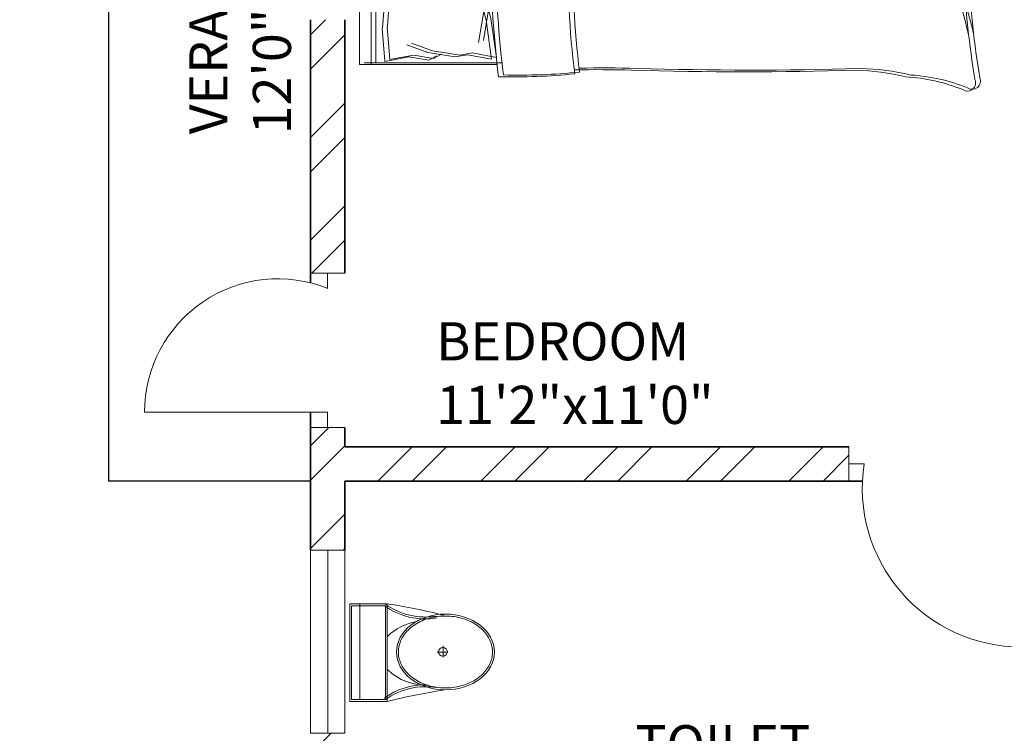
# Model space of a CAD drawing. Units: inches. Extents: x 1885 to 2748, y 783 to 2421.
# Tile 30 of 117: x 1969 to 2098, y 1350 to 1443. Entities that reach past the tile are written whole.
import ezdxf

# ---------------------------------------------------------------- set-up
doc = ezdxf.new("R2010")
doc.units = ezdxf.units.IN
for name, color, linetype, lineweight in [('A-ANNO-DIMS', 2, 'Continuous', 18), ('A-AREA-IDEN', 7, 'Continuous', 18), ('A-DOOR', 31, 'Continuous', 18), ('A-FLOR-BALC', 7, 'Continuous', 25), ('A-FLOR-FIXT', 8, 'Continuous', 18), ('A-FURN', 8, 'Continuous', 13), ('A-GLAZ', 181, 'Continuous', 18), ('A-WALL', 7, 'Continuous', 35)]:
    doc.layers.add(name, color=color, linetype=linetype, lineweight=lineweight)
doc.layers.add('A-WALL-PATT', color=85, linetype='Continuous', lineweight=13, true_color=0x58ba48)
doc.styles.get("Standard").update_dxf_attribs({"font": 'arial.ttf'})
doc.dimstyles.get("Standard").update_dxf_attribs({"dimtxt": 0.18, "dimasz": 0.18, "dimexe": 0.18, "dimexo": 0.0625, "dimgap": 0.09, "dimtad": 0, "dimtih": 1, "dimtoh": 1, "dimdec": 4, "dimzin": 0, "dimdsep": 46, "dimtxsty": 'Standard', "dimcen": 0.09, "dimadec": 0, "dimazin": 0, "dimtfac": 1, "dimtdec": 4, "dimtofl": 0, "dimtmove": 0, "dimatfit": 3, "dimfxl": 1, "dimtolj": 1, "dimtzin": 0, "dimarcsym": 0})

# ---------------------------------------------------------------- blocks, each defined once
blk = doc.blocks.new('A$C31115884')
for p, q in [((283.1, 497.7), (223.4, 497.7)), ((257.5, 466.4), (257.5, 523.2)), ((0, 200), (0, 0)), ((520, 200), (0, 200)), ((10, 190), (10, 10)), ((510, 190), (10, 190)), ((510, 10), (510, 190)), ((520, 0), (520, 200)), ((510, 54.5), (0, 54.5)), ((10, 10), (510, 10)), ((0, 0), (520, 0))]:
    blk.add_line(p, q)
blk.add_circle((255.6, 496.4), 23.6)
for centre, radius, start, end in [((2777.7, -204.6), 2807, 165.4549, 171.7133), ((3237, 905), 2807, 188.2867, 194.5451), ((-294.5, 403.3), 364.7, 324.2091, 9.3499), ((-294.5, 403.3), 374.7, 324.2091, 9.3499), ((139.5, 406.2), 293.5, 315.8436, 2.6563), ((805.8, 403.3), 364.7, 170.6501, 215.7909), ((805.8, 403.3), 374.7, 179.2036, 215.7909), ((383.6, 406.2), 293.5, 190.2774, 224.1564)]:
    blk.add_arc(centre, radius, start, end)
blk.add_ellipse((256.2, 509.9), major_axis=(0, -260.7), ratio=0.772727)
blk.add_open_spline([(256.2, 259.2), (263.1, 259.2), (270, 259.7), (287.8, 262.3), (298.7, 265.1), (319.9, 273.1), (330.2, 278.4), (350.1, 291.1), (359.7, 298.7), (377.7, 315.9), (386.2, 325.5), (401.7, 346.6), (408.8, 358.1), (421.3, 382.5), (426.8, 395.5), (435.9, 422.4), (439.5, 436.4), (444.8, 465.1), (446.5, 479.7), (447.9, 509.2), (447.6, 524), (445, 553.3), (442.7, 567.8), (436.3, 596), (432.1, 609.7), (421.9, 636), (416, 648.6), (402.5, 672.1), (395, 683), (378.6, 703), (369.8, 712.1), (351.1, 728), (341.3, 734.8), (320.9, 746.2), (310.4, 750.7), (288.9, 757.3), (278, 759.4), (256, 761), (245, 760.6), (223.1, 757.2), (212.3, 754.3), (191.1, 746.1), (180.8, 740.7), (160.9, 727.8), (151.4, 720.1), (133.5, 702.7), (125.1, 693), (109.6, 671.7), (102.6, 660.2), (90.2, 635.7), (84.9, 622.7), (76, 595.6), (72.4, 581.6), (67.2, 552.9), (65.6, 538.2), (64.4, 508.8), (64.8, 494), (67.5, 464.7), (69.9, 450.2), (76.6, 422), (80.8, 408.3), (91.1, 382.2), (97.2, 369.7), (110.8, 346.3), (118.4, 335.4), (134.8, 315.6), (143.7, 306.7), (162.4, 290.9), (172.3, 284.2), (192.8, 273), (203.3, 268.6), (224.8, 262.2), (235.8, 260.2), (249.9, 259.3), (253, 259.2), (256.2, 259.2)], degree=3, knots=[0, 0, 0, 0, 0.110105, 0.110105, 0.285049, 0.285049, 0.459994, 0.459994, 0.634938, 0.634938, 0.809882, 0.809882, 0.984827, 0.984827, 1.159771, 1.159771, 1.334715, 1.334715, 1.50966, 1.50966, 1.684604, 1.684604, 1.859549, 1.859549, 2.034493, 2.034493, 2.209437, 2.209437, 2.384382, 2.384382, 2.559326, 2.559326, 2.73427, 2.73427, 2.909215, 2.909215, 3.084159, 3.084159, 3.259103, 3.259103, 3.434048, 3.434048, 3.608992, 3.608992, 3.783936, 3.783936, 3.958881, 3.958881, 4.133825, 4.133825, 4.30877, 4.30877, 4.483714, 4.483714, 4.658658, 4.658658, 4.833603, 4.833603, 5.008547, 5.008547, 5.183491, 5.183491, 5.358436, 5.358436, 5.53338, 5.53338, 5.708324, 5.708324, 5.883269, 5.883269, 6.058213, 6.058213, 6.233158, 6.233158, 6.283185, 6.283185, 6.283185, 6.283185])
blk = doc.blocks.new('BED-DOUBLE')
for p, q in [((28.39, 53.09), (25.14, 49.39)), ((28.39, 53.09), (25.14, 49.39)), ((29.49, 52.95), (27.75, 52.87, 3.87)), ((29.49, 52.95), (27.75, 52.87, 3.87)), ((30.13, 53.17), (28.39, 53.09, 3.87)), ((30.13, 53.17), (28.39, 53.09, 3.87)), ((29.01, 51.56), (28.39, 53.09)), ((29.01, 51.56), (28.39, 53.09)), ((27.75, 52.87), (24.5, 49.16)), ((27.75, 52.87), (24.5, 49.16)), ((28.37, 51.33), (27.75, 52.87)), ((28.37, 51.33), (27.75, 52.87)), ((0, 51.49), (0.64, 51.49)), ((0, 3.47), (0, 51.49)), ((0, 51.26), (26.61, 51.26)), ((0, 51.26), (26.61, 51.26)), ((0.64, 51.49), (27.25, 51.49)), ((0.64, 51.49), (27.25, 51.49)), ((1.54, 3.47), (1.54, 51.26)), ((1.54, 3.47), (1.54, 51.26)), ((2.18, 3.7), (2.18, 51.49)), ((2.18, 3.7), (2.18, 51.49)), ((6.41, 49.96), (8.98, 50.56)), ((6.41, 49.96), (8.98, 50.56)), ((8.98, 50.56), (10.03, 50.04)), ((8.98, 50.56), (10.03, 50.04)), ((16.58, 50.7), (13.44, 49.92)), ((16.58, 50.7), (13.44, 49.92)), ((17.22, 50.93), (14.08, 50.15)), ((17.22, 50.93), (14.08, 50.15)), ((16.17, 45.57), (16.58, 50.7)), ((16.17, 45.56), (16.58, 50.7)), ((16.81, 45.79), (17.22, 50.93)), ((16.81, 45.79), (17.22, 50.93)), ((28.06, 48.23), (28.37, 51.33)), ((28.06, 48.23), (28.37, 51.33)), ((28.7, 48.46), (29.01, 51.56)), ((28.7, 48.46), (29.01, 51.56)), ((2.56, 50.11), (2.46, 44.71)), ((2.56, 50.11), (2.46, 44.71)), ((2.56, 50.11), (5.77, 49.73)), ((2.56, 50.11), (5.77, 49.73)), ((3.2, 50.34), (3.1, 44.94)), ((3.2, 50.34), (3.1, 44.94)), ((3.2, 50.34), (6.41, 49.96)), ((3.2, 50.34), (6.41, 49.96)), ((8.26, 49.31), (5.58, 48.13)), ((8.26, 49.31), (5.58, 48.13)), ((5.77, 49.73), (8.34, 50.33)), ((5.77, 49.73), (8.34, 50.33)), ((8.9, 49.54), (6.22, 48.36)), ((8.9, 49.54), (6.22, 48.36)), ((11.83, 50.11), (8.26, 49.31)), ((11.83, 50.11), (8.26, 49.31)), ((8.34, 50.33), (9.39, 49.81)), ((8.34, 50.33), (9.39, 49.81)), ((12.47, 50.34), (8.9, 49.54)), ((12.47, 50.34), (8.9, 49.54)), ((13.44, 49.92), (11.83, 50.11)), ((13.44, 49.92), (11.83, 50.11)), ((14.08, 50.15), (12.47, 50.34)), ((14.08, 50.15), (12.47, 50.34)), ((24.5, 49.16), (22.33, 46.22)), ((24.5, 49.16), (22.33, 46.22)), ((25.14, 49.39), (22.97, 46.45)), ((25.14, 49.39), (22.97, 46.45)), ((28.37, 44.36), (28.06, 48.23)), ((28.37, 44.36), (28.06, 48.23)), ((29.01, 44.59), (28.7, 48.46)), ((29.01, 44.59), (28.7, 48.46)), ((2.46, 44.71), (2.55, 45.71)), ((2.46, 44.71), (2.55, 45.71)), ((2.55, 45.71), (3.07, 41.91)), ((2.55, 45.71), (3.07, 41.91)), ((3.1, 44.94), (3.19, 45.94)), ((3.1, 44.94), (3.19, 45.94)), ((3.19, 45.94), (3.71, 42.14)), ((3.19, 45.94), (3.71, 42.14)), ((16.73, 43.6), (16.17, 45.57)), ((16.73, 43.6), (16.17, 45.56)), ((17.37, 43.83), (16.81, 45.79)), ((17.37, 43.83), (16.81, 45.79)), ((22.33, 46.22), (20.32, 40.64)), ((22.33, 46.22), (20.32, 40.64)), ((22.97, 46.45), (20.96, 40.87)), ((22.97, 46.45), (20.96, 40.87)), ((28.83, 40.95), (28.37, 44.36)), ((28.83, 40.95), (28.37, 44.36)), ((29.47, 41.18), (29.01, 44.59)), ((29.47, 41.18), (29.01, 44.59)), ((16.3, 36.59), (16.73, 43.6)), ((16.3, 36.59), (16.73, 43.6)), ((16.94, 36.82), (17.37, 43.83)), ((16.94, 36.82), (17.37, 43.83)), ((3.07, 41.91), (4.43, 36.49)), ((3.07, 41.91), (4.43, 36.49)), ((3.71, 42.14), (5.07, 36.72)), ((3.71, 42.14), (5.07, 36.72)), ((20.32, 40.64), (17.39, 32.3)), ((20.32, 40.64), (17.39, 32.3)), ((20.96, 40.87), (18.03, 32.53)), ((20.96, 40.87), (18.03, 32.53)), ((29.76, 38.94), (28.83, 40.95)), ((29.76, 38.94), (28.83, 40.95)), ((30.4, 39.17), (29.47, 41.18)), ((30.4, 39.17), (29.47, 41.18)), ((3.68, 39.2), (3.08, 37.13)), ((3.68, 39.2), (3.08, 37.13)), ((4.32, 39.43), (3.72, 37.36)), ((4.32, 39.43), (3.72, 37.36)), ((30.38, 36.46), (29.76, 38.94)), ((30.38, 36.46), (29.76, 38.94)), ((31.02, 36.69), (30.4, 39.17)), ((31.02, 36.69), (30.4, 39.17)), ((79.25, 15.06), (79.25, 39.68)), ((79.25, 15.06), (79.25, 39.68)), ((79.89, 15.29), (79.89, 39.9)), ((79.89, 15.29), (79.89, 39.9)), ((3.08, 37.13), (2.54, 34.2)), ((3.08, 37.13), (2.54, 34.2)), ((3.72, 37.36), (3.18, 34.43)), ((3.72, 37.36), (3.18, 34.43)), ((15.63, 32.56), (16.3, 36.59)), ((15.63, 32.56), (16.3, 36.59)), ((16.27, 32.79), (16.94, 36.82)), ((16.27, 32.79), (16.94, 36.82)), ((23.88, 34.45), (28.37, 36.15)), ((23.88, 34.45), (28.37, 36.15)), ((24.52, 34.68), (29.01, 36.38)), ((24.52, 34.68), (29.01, 36.38)), ((28.37, 36.15), (30.38, 36.46)), ((28.37, 36.15), (30.38, 36.46)), ((29.01, 36.38), (31.02, 36.69)), ((29.01, 36.38), (31.02, 36.69)), ((2.54, 34.2), (2.56, 33.88)), ((2.54, 34.2), (2.56, 33.88)), ((2.56, 33.88), (2.98, 29.45)), ((2.56, 33.88), (2.98, 29.45)), ((3.18, 34.43), (3.2, 34.11)), ((3.18, 34.43), (3.2, 34.11)), ((3.2, 34.11), (3.62, 29.68)), ((3.2, 34.11), (3.62, 29.68)), ((16.74, 30.75), (15.46, 33.82)), ((16.74, 30.75), (15.46, 33.82)), ((17.38, 30.98), (16.1, 34.05)), ((17.38, 30.98), (16.1, 34.05)), ((17.39, 30.26), (23.88, 34.45)), ((17.39, 30.26), (23.88, 34.45)), ((18.03, 30.49), (24.52, 34.68)), ((18.03, 30.49), (24.52, 34.68)), ((16.9, 28.3), (16.74, 30.75)), ((16.9, 28.3), (16.74, 30.75)), ((17.54, 28.52), (17.38, 30.98)), ((17.54, 28.52), (17.38, 30.98)), ((2.98, 29.45), (2.5, 27.98)), ((2.98, 29.45), (2.5, 27.98)), ((3.62, 29.68), (3.13, 28.2)), ((3.62, 29.68), (3.13, 28.2)), ((14.86, 28.36), (17.54, 28.52)), ((14.86, 28.36), (17.54, 28.52)), ((2.5, 27.98), (7.87, 27.73)), ((2.5, 27.98), (7.87, 27.73)), ((3.13, 28.2), (8.51, 27.96)), ((3.13, 28.2), (8.51, 27.96)), ((7.22, 26.56), (10.4, 27.14)), ((7.22, 26.56), (10.4, 27.14)), ((7.86, 26.79), (11.04, 27.37)), ((7.86, 26.79), (11.04, 27.37)), ((7.87, 27.73), (11.08, 27.35)), ((7.87, 27.73), (11.08, 27.35)), ((8.51, 27.96), (11.72, 27.58)), ((8.51, 27.96), (11.72, 27.58)), ((10.4, 27.14), (11.71, 27.14)), ((10.4, 27.14), (11.71, 27.14)), ((11.04, 27.37), (12.35, 27.37)), ((11.04, 27.37), (12.35, 27.37)), ((11.08, 27.35), (12.38, 27.43)), ((11.08, 27.35), (12.38, 27.43)), ((11.71, 27.14), (13.59, 26.56)), ((11.71, 27.14), (13.59, 26.56)), ((11.72, 27.58), (13.02, 27.66)), ((11.72, 27.58), (13.02, 27.66)), ((12.35, 27.37), (14.22, 26.79)), ((12.35, 27.37), (14.22, 26.79)), ((12.38, 27.43), (14.22, 28.13)), ((12.38, 27.43), (14.22, 28.13)), ((13.02, 27.66), (14.86, 28.36)), ((13.02, 27.66), (14.86, 28.36)), ((14.22, 28.13), (16.9, 28.3)), ((14.22, 28.13), (16.9, 28.3)), ((1.87, 25.98), (7.22, 26.56)), ((1.87, 25.98), (7.22, 26.56)), ((2.45, 24.54), (1.87, 25.98)), ((2.45, 24.54), (1.87, 25.98)), ((2.51, 26.21), (7.86, 26.79)), ((2.51, 26.21), (7.86, 26.79)), ((3.09, 24.76), (2.51, 26.21)), ((3.09, 24.76), (2.51, 26.21)), ((13.59, 26.56), (16.27, 26.56)), ((13.59, 26.56), (16.27, 26.56)), ((14.22, 26.79), (16.91, 26.79)), ((14.22, 26.79), (16.91, 26.79)), ((16.27, 26.56), (16.27, 24.1)), ((16.27, 26.56), (16.27, 24.1)), ((16.91, 26.79), (16.91, 24.33)), ((16.91, 26.79), (16.91, 24.33)), ((2.31, 20.09), (2.45, 24.54)), ((2.31, 20.09), (2.45, 24.54)), ((2.95, 20.32), (3.09, 24.76)), ((2.95, 20.32), (3.09, 24.76)), ((16.81, 19.61), (17.22, 24.74)), ((16.81, 19.61), (17.22, 24.74)), ((16.27, 24.1), (15.18, 20.96)), ((16.27, 24.1), (15.18, 20.96)), ((16.91, 24.33), (15.82, 21.19)), ((16.91, 24.33), (15.82, 21.19)), ((16.17, 19.38), (16.58, 24.51)), ((16.17, 19.38), (16.58, 24.51)), ((2.31, 19.77), (2.31, 20.09)), ((2.31, 19.77), (2.31, 20.09)), ((3.03, 16.88), (2.31, 19.77)), ((3.03, 16.88), (2.31, 19.77)), ((2.95, 20), (2.95, 20.32)), ((2.95, 20), (2.95, 20.32)), ((3.67, 17.11), (2.95, 20)), ((3.67, 17.11), (2.95, 20)), ((16.73, 17.42), (16.17, 19.38)), ((16.73, 17.42), (16.17, 19.38)), ((17.37, 17.65), (16.81, 19.61)), ((17.37, 17.65), (16.81, 19.61)), ((3.75, 14.85), (3.03, 16.88)), ((3.75, 14.85), (3.03, 16.88)), ((3.32, 12.11), (4.33, 17.6)), ((3.32, 12.11), (4.33, 17.6)), ((4.39, 15.08), (3.67, 17.11)), ((4.39, 15.08), (3.67, 17.11)), ((3.96, 12.34), (4.97, 17.83)), ((3.96, 12.34), (4.97, 17.83)), ((16.3, 10.41), (16.73, 17.42)), ((16.3, 10.41), (16.73, 17.42)), ((16.94, 10.64), (17.37, 17.65)), ((16.94, 10.64), (17.37, 17.65)), ((3.03, 8.28), (3.32, 12.11)), ((3.03, 8.28), (3.32, 12.11)), ((3.67, 8.51), (3.96, 12.34)), ((3.67, 8.51), (3.96, 12.34)), ((15.63, 6.38), (16.3, 10.41)), ((15.63, 6.38), (16.3, 10.41)), ((16.27, 6.61), (16.94, 10.64)), ((16.27, 6.61), (16.94, 10.64)), ((16.3, 10.41), (16.62, 9.28)), ((16.3, 10.41), (16.62, 9.28)), ((16.94, 10.64), (17.26, 9.51)), ((16.94, 10.64), (17.26, 9.51)), ((16.62, 9.28), (17.34, 4.18)), ((16.62, 9.28), (17.34, 4.18)), ((17.26, 9.51), (17.98, 4.41)), ((17.26, 9.51), (17.98, 4.41)), ((3.01, 8.18), (3.03, 8.28)), ((3.01, 8.18), (3.03, 8.28)), ((3.34, 3.9), (3.01, 8.18)), ((3.34, 3.9), (3.01, 8.18)), ((3.65, 8.41), (3.67, 8.51)), ((3.65, 8.41), (3.67, 8.51)), ((3.98, 4.13), (3.65, 8.41)), ((3.98, 4.13), (3.65, 8.41)), ((8.96, 5.05), (6.21, 6.06)), ((8.96, 5.05), (6.21, 6.06)), ((9.6, 5.28), (6.85, 6.29)), ((9.6, 5.28), (6.85, 6.29)), ((13.21, 4.7), (9.6, 5.28)), ((13.21, 4.7), (9.6, 5.28)), ((3.32, 3.89), (6.5, 4.47)), ((3.32, 3.89), (6.5, 4.47)), ((3.96, 4.12), (7.14, 4.7)), ((3.96, 4.12), (7.14, 4.7)), ((6.5, 4.47), (9.1, 4.04)), ((6.5, 4.47), (9.1, 4.04)), ((7.14, 4.7), (9.74, 4.27)), ((7.14, 4.7), (9.74, 4.27)), ((12.57, 4.47), (8.96, 5.05)), ((12.57, 4.47), (8.96, 5.05)), ((9.1, 4.04), (10.12, 4.62)), ((9.1, 4.04), (10.12, 4.62)), ((9.74, 4.27), (10.75, 4.84)), ((9.74, 4.27), (10.75, 4.84)), ((14.16, 4.76), (12.57, 4.47)), ((14.16, 4.76), (12.57, 4.47)), ((14.8, 4.99), (13.21, 4.7)), ((14.8, 4.99), (13.21, 4.7)), ((17.34, 4.18), (14.16, 4.76)), ((17.34, 4.18), (14.16, 4.76)), ((17.98, 4.41), (14.8, 4.99)), ((17.98, 4.41), (14.8, 4.99)), ((18.11, 3.47), (0, 3.47)), ((18.11, 3.47), (0, 3.47)), ((18.75, 3.7), (0.64, 3.7)), ((18.75, 3.7), (0.64, 3.7))]:
    blk.add_line(p, q)
for centre, radius, start, end in [((69.31, 76.38), 23.07, 267.4714, 296.4681), ((69.31, 76.38), 23.07, 267.4714, 296.4681), ((79.51, 54.64), 1.1, 332.6588, 86.02), ((79.51, 54.64), 1.1, 332.6588, 86.02), ((68.67, 76.16), 23.07, 267.4714, 296.4681), ((68.67, 76.16), 23.07, 267.4714, 296.4681), ((78.87, 54.41), 1.1, 332.6588, 86.02), ((78.87, 54.41), 1.1, 332.6588, 86.02), ((-6.65, 51.33), 36.18, 349.8763, 2.5657), ((-6.65, 51.33), 36.18, 349.8763, 2.5657), ((36.32, 182.26), 129.5, 266.9791, 273.8365), ((36.32, 182.26), 129.5, 266.9791, 273.8365), ((-6.01, 51.55), 36.18, 349.8763, 2.5657), ((-6.01, 51.55), 36.18, 349.8763, 2.5657), ((36.96, 182.49), 129.5, 266.9791, 273.8365), ((36.96, 182.49), 129.5, 266.9791, 273.8365), ((67.83, -4508.74), 4561.86, 90.00217, 90.28689), ((67.83, -4508.75), 4561.86, 90.00217, 90.28689), ((68.46, -4508.52), 4561.86, 90.00217, 90.28689), ((68.46, -4508.52), 4561.86, 90.00217, 90.28689), ((212.28, 41.15), 133.04, 174.4998, 180.6351), ((212.28, 41.15), 133.04, 174.4998, 180.6351), ((212.92, 41.38), 133.04, 174.4998, 180.6351), ((212.92, 41.38), 133.04, 174.4998, 180.6351), ((35.71, 43.97), 6.22, 168.6608, 203.7384), ((35.71, 43.97), 6.22, 168.6608, 203.7384), ((35.07, 43.74), 6.22, 168.6608, 203.7384), ((35.07, 43.74), 6.22, 168.6608, 203.7384), ((2.13, 31.38), 29.65, 10.6617, 19.8806), ((2.13, 31.38), 29.65, 10.6617, 19.8806), ((1.49, 31.15), 29.65, 10.6617, 19.8806), ((1.49, 31.15), 29.65, 10.6617, 19.8806), ((156.32, 17.75), 129.02, 171.7845, 186.9006), ((156.32, 17.75), 129.02, 171.7845, 186.9006), ((156.96, 17.98), 129.02, 171.7845, 186.9006), ((156.96, 17.98), 129.02, 171.7845, 186.9006), ((30.44, 36.64), 0.185, 250.2464, 1.1377), ((30.44, 36.63), 0.185, 250.2464, 1.1377), ((31.08, 36.86), 0.185, 250.2464, 1.1377), ((31.08, 36.86), 0.185, 250.2464, 1.1377), ((182.06, 21.36), 164.97, 176.0865, 186.7821), ((182.06, 21.36), 164.97, 176.0865, 186.7821), ((182.7, 21.59), 164.97, 176.0865, 186.7821), ((182.7, 21.59), 164.97, 176.0865, 186.7821), ((-23.71, -17.22), 106.46, 13.3832, 17.7053), ((-23.71, -17.22), 106.46, 13.3832, 17.7053), ((-23.07, -16.99), 106.46, 13.3832, 17.7053), ((-23.07, -16.99), 106.46, 13.3832, 17.7053), ((200.84, 21.43), 121.76, 182.9958, 189.4091), ((200.84, 21.43), 121.76, 182.9958, 189.4091), ((201.48, 21.65), 121.76, 182.9958, 189.4091), ((201.48, 21.65), 121.76, 182.9958, 189.4091), ((31.18, -167.31), 170.11, 88.4762, 91.0082), ((31.18, -167.31), 170.11, 88.4762, 91.0082), ((31.82, -167.08), 170.11, 88.4762, 91.0082), ((31.82, -167.08), 170.11, 88.4762, 91.0082), ((50.62, 484.82), 482.31, 268.2277, 271.7185), ((50.62, 484.82), 482.31, 268.2277, 271.7185), ((51.26, 485.05), 482.31, 268.2277, 271.7185), ((51.26, 485.05), 482.31, 268.2277, 271.7185), ((64.52, -26.9), 29.63, 76.0648, 88.9113), ((64.52, -26.9), 29.63, 76.0648, 88.9113), ((65.16, -26.67), 29.63, 76.0648, 88.9113), ((65.16, -26.67), 29.63, 76.0648, 88.9113), ((20.1, 85.16), 83.31, 268.7218, 275.604), ((20.1, 85.16), 83.31, 268.7218, 275.604), ((20.74, 85.39), 83.31, 268.7218, 275.604), ((20.74, 85.39), 83.31, 268.7218, 275.604), ((70.28, -21.66), 23.56, 67.9751, 86.652), ((70.28, -21.66), 23.56, 67.9751, 86.652), ((70.92, -21.43), 23.56, 67.9751, 86.652), ((70.92, -21.43), 23.56, 67.9751, 86.652), ((79.72, 1.09), 1.09, 236.1736, 23.4781), ((79.72, 1.09), 1.09, 236.1736, 23.4781), ((80.36, 1.31), 1.09, 236.1736, 23.4781), ((80.36, 1.31), 1.09, 236.1736, 23.4781)]:
    blk.add_arc(centre, radius, start, end)
blk = doc.blocks.new('WIN-24')
for p, q in [((0, 4.5), (0, 0)), ((0, 4.5), (24, 4.5)), ((24, 2.25), (24, 4.5)), ((24, 4.5), (24, 0)), ((0, 0), (0, 2.25)), ((0, 2.25), (24, 2.25)), ((24, 0), (0, 0))]:
    blk.add_line(p, q)
blk = doc.blocks.new('*D45')
at = {"layer": 'A-ANNO-DIMS', "color": 0, "lineweight": -2, "transparency": 16777216}
for p, q in [((1980.71, 1524.01), (1902.84, 1524.01)), ((1903.02, 1523.83), (1903.02, 1290.94)), ((1903.02, 1057.69), (1903.02, 1290.57)), ((1971.21, 1057.51), (1902.84, 1057.51))]:
    blk.add_line(p, q, dxfattribs=at)
at = {"layer": 'A-ANNO-DIMS', "color": 0, "transparency": 16777216}
for points in [[(1902.99, 1523.83), (1903.05, 1523.83), (1903.02, 1524.01)], [(1902.99, 1057.69), (1903.05, 1057.69), (1903.02, 1057.51)]]:
    blk.add_solid(points, dxfattribs=at)
at = {"layer": 'Defpoints', "color": 0, "transparency": 16777216}
for p in [(1903.02, 1524.01), (1980.77, 1524.01), (1971.27, 1057.51)]:
    blk.add_point(p, dxfattribs=at)
at = {"layer": 'A-ANNO-DIMS', "color": 0, "transparency": 16777216, "insert": (1903.02, 1290.76), "char_height": 0.18, "attachment_point": 5}
blk.add_mtext('\\A1;466.5', dxfattribs=at)

msp = doc.modelspace()

# ---------------------------------------------------------------- hatches: boundary and pattern name
at = {"layer": 'A-WALL-PATT'}
h = msp.add_hatch(dxfattribs=at)
h.set_pattern_fill('ANSI32', color=256)
h.paths.add_polyline_path([(2007.77, 2318.01), (1980.77, 2318.01), (1980.77, 2281.22), (1985.27, 2281.22), (1985.27, 2313.51), (2007.77, 2313.51), (2007.77, 2315.76)])
h.paths.add_polyline_path([(2094.32, 2318.01), (2067.77, 2318.01), (2067.77, 2313.51), (2094.32, 2313.51), (2094.32, 2315.76)])
h.paths.add_polyline_path([(2131.37, 2315.76), (2131.37, 2318.01), (2131.19, 2318.01), (2112.61, 2318.01), (2112.61, 2313.51), (2117.27, 2313.51), (2117.27, 2255.2), (2121.77, 2255.2), (2121.77, 2313.51), (2131.37, 2313.51)])
h.paths.add_polyline_path([(2190.51, 2318.01), (2155.37, 2318.01), (2155.37, 2313.51), (2169.77, 2313.51), (2169.77, 2229.51), (2121.77, 2229.51), (2121.77, 2233.45), (2119.52, 2233.45), (2117.27, 2233.45), (2117.27, 2201.1), (2121.77, 2201.1), (2121.77, 2225.01), (2169.77, 2225.01), (2169.77, 2165.01), (2306.27, 2165.01), (2306.27, 2066.01), (2310.77, 2066.01), (2344.27, 2066.01), (2486.27, 2066.01), (2486.27, 1886.01), (2483.02, 1886.01), (2483.02, 1881.51), (2486.27, 1881.51), (2486.27, 1880.68), (2490.77, 1880.68), (2490.77, 2070.51), (2344.27, 2070.51), (2310.77, 2070.51), (2310.77, 2165.01), (2310.77, 2173.64), (2308.52, 2173.64), (2306.27, 2173.64), (2306.27, 2169.51), (2174.27, 2169.51), (2174.27, 2313.51), (2190.51, 2313.51), (2190.51, 2315.76)])
h.paths.add_polyline_path([(1985.27, 2221.22), (1980.77, 2221.22), (1980.77, 2165.01), (1992.77, 2165.01), (1992.77, 2141.93), (1997.27, 2141.93), (1997.27, 2165.01), (2117.27, 2165.01), (2117.27, 2163.13), (2121.77, 2163.13), (2121.77, 2172.73), (2119.52, 2172.73), (2117.27, 2172.73), (2117.27, 2169.51), (1985.27, 2169.51)])
h.paths.add_polyline_path([(1997.27, 2105.93), (1992.77, 2105.93), (1992.77, 2070.51), (2016.77, 2070.51), (2016.77, 2059.12), (2019.02, 2059.12), (2021.27, 2059.12), (2021.27, 2070.51), (2117.27, 2070.51), (2117.27, 2022.51), (2114.42, 2022.51), (2114.42, 2018.01), (2123.63, 2018.01), (2123.63, 2020.26), (2123.63, 2022.51), (2121.77, 2022.51), (2121.77, 2142.59), (2119.52, 2142.59), (2117.27, 2142.59), (2117.27, 2075.01), (1997.27, 2075.01)])
h.paths.add_polyline_path([(2092.03, 2020.26), (2092.03, 2022.51), (2021.27, 2022.51), (2021.27, 2035.12), (2016.77, 2035.12), (2016.77, 2018.01), (2016.77, 1978.78), (2021.27, 1978.78), (2021.27, 2018.01), (2092.03, 2018.01)])
h.paths.add_polyline_path([(2260.94, 2022.51), (2153.1, 2022.51), (2153.1, 2020.26), (2153.1, 2018.01), (2155.27, 2018.01), (2155.27, 1886.01), (2107.63, 1886.01), (2107.63, 1881.51), (2182.91, 1881.51), (2182.91, 1883.76), (2182.91, 1886.01), (2159.77, 1886.01), (2159.77, 2018.01), (2260.94, 2018.01), (2260.94, 2020.26)])
h.paths.add_polyline_path([(2047.63, 1883.76), (2047.63, 1886.01), (2021.27, 1886.01), (2021.27, 1918.78), (2019.02, 1918.78), (2016.77, 1918.78), (2016.77, 1881.51), (2047.63, 1881.51)])
h.paths.add_polyline_path([(2306.36, 1883.76), (2306.36, 1886.01), (2296.27, 1886.01), (2296.27, 1982.01), (2316.54, 1982.01), (2316.54, 1984.26), (2316.54, 1986.51), (2296.27, 1986.51), (2296.27, 2022.51), (2289.28, 2022.51), (2289.28, 2018.01), (2291.77, 2018.01), (2291.77, 1886.01), (2242.91, 1886.01), (2242.91, 1881.51), (2306.36, 1881.51)], flags=17)
h.paths.add_polyline_path([(1985.27, 1843.01), (2021.6, 1843.01), (2021.53, 1845.44), (2021.48, 1847.51), (1980.77, 1847.51), (1980.77, 1809.45), (1985.27, 1809.45)])
h.paths.add_polyline_path([(2131.48, 1845.26), (2131.48, 1847.51), (2081.53, 1847.51), (2081.53, 1843.01), (2117.27, 1843.01), (2117.27, 1784.15), (2119.52, 1784.15), (2121.77, 1784.15), (2121.77, 1843.01), (2131.48, 1843.01)])
h.paths.add_polyline_path([(2203.89, 1847.51), (2155.48, 1847.51), (2155.48, 1843.01), (2169.77, 1843.01), (2169.77, 1759.01), (2121.77, 1759.01), (2121.77, 1761.46), (2117.27, 1761.46), (2117.27, 1730.43), (2121.77, 1730.43), (2121.77, 1754.51), (2177.42, 1754.51), (2177.42, 1756.76), (2177.42, 1759.01), (2174.27, 1759.01), (2174.27, 1843.01), (2203.89, 1843.01)])
h.paths.add_polyline_path([(2335.55, 1845.26), (2335.55, 1847.51), (2239.89, 1847.51), (2239.89, 1843.01), (2306.27, 1843.01), (2306.27, 1759.01), (2199.49, 1759.01), (2199.49, 1754.51), (2310.77, 1754.51), (2310.77, 1843.01), (2335.55, 1843.01)])
h.paths.add_polyline_path([(2348.77, 2022.51), (2344.27, 2022.51), (2344.27, 1986.51), (2341.68, 1986.51), (2341.68, 1982.01), (2344.27, 1982.01), (2344.27, 1886.01), (2330.36, 1886.01), (2330.36, 1881.51), (2361.63, 1881.51), (2361.63, 1883.76), (2361.63, 1886.01), (2348.77, 1886.01)], flags=17)
h.paths.add_polyline_path([(2283.25, 2315.76), (2283.25, 2318.01), (2238.51, 2318.01), (2238.51, 2313.51), (2283.25, 2313.51)], flags=17)
h.paths.add_polyline_path([(2363.27, 2348.01), (2388.68, 2348.01), (2388.68, 2350.26), (2388.68, 2352.51), (2358.77, 2352.51), (2358.77, 2348.01), (2358.77, 2318.01), (2344.48, 2318.01), (2344.48, 2313.51), (2358.77, 2313.51), (2358.77, 2229.51), (2310.77, 2229.51), (2310.77, 2231.95), (2306.27, 2231.95), (2306.27, 2205.61), (2310.77, 2205.61), (2310.77, 2225.01), (2358.77, 2225.01), (2358.77, 2211.51), (2452.33, 2211.51), (2452.33, 2213.76), (2452.33, 2216.01), (2363.27, 2216.01), (2363.27, 2318.01)])
h.paths.add_polyline_path([(2310.77, 2313.51), (2320.48, 2313.51), (2320.48, 2315.76), (2320.48, 2318.01), (2302.73, 2318.01), (2302.73, 2313.51), (2306.27, 2313.51), (2306.27, 2251.08), (2310.77, 2251.08)], flags=17)
h.paths.add_polyline_path([(2490.77, 2352.51), (2486.27, 2352.51), (2448.68, 2352.51), (2448.68, 2348.01), (2486.27, 2348.01), (2486.27, 2318.01), (2486.27, 2216.01), (2481.78, 2216.01), (2481.78, 2211.51), (2486.27, 2211.51), (2486.27, 2165.01), (2493.29, 2165.01), (2493.29, 2167.26), (2493.29, 2169.51), (2490.77, 2169.51), (2490.77, 2313.51), (2494.43, 2313.51), (2494.43, 2318.01), (2490.77, 2318.01)])
h.paths.add_polyline_path([(2534.65, 2318.01), (2515.69, 2318.01), (2515.69, 2313.51), (2534.65, 2313.51), (2534.65, 2315.76)])
h.paths.add_polyline_path([(2618.27, 2318.01), (2594.65, 2318.01), (2594.65, 2313.51), (2613.77, 2313.51), (2613.77, 2281.71), (2618.27, 2281.71)])
h.paths.add_polyline_path([(2618.27, 2221.71), (2613.77, 2221.71), (2613.77, 2169.51), (2554.02, 2169.51), (2554.02, 2165.01), (2613.77, 2165.01), (2613.77, 2152.88), (2618.27, 2152.88)])
h.paths.add_polyline_path([(2618.27, 2128.88), (2616.02, 2128.88), (2613.77, 2128.88), (2613.77, 2117.01), (2529.77, 2117.01), (2529.77, 2165.01), (2532.85, 2165.01), (2532.85, 2169.51), (2522.87, 2169.51), (2522.87, 2165.01), (2525.27, 2165.01), (2525.27, 2117.01), (2525.27, 2112.51), (2525.27, 2108.58), (2529.77, 2108.58), (2529.77, 2112.51), (2613.77, 2112.51), (2613.77, 2080.19), (2618.27, 2080.19)])
h.paths.add_polyline_path([(2618.27, 2044.19), (2616.02, 2044.19), (2613.77, 2044.19), (2613.77, 2015.51), (2529.77, 2015.51), (2529.77, 2088.58), (2527.52, 2088.58), (2525.27, 2088.58), (2525.27, 2011.01), (2613.77, 2011.01), (2613.77, 1956.75), (2618.27, 1956.75)])
h.paths.add_polyline_path([(2618.27, 1881.51), (2618.27, 1896.75), (2613.77, 1896.75), (2613.77, 1881.51), (2613.77, 1847.51), (2592.71, 1847.51), (2592.71, 1843.01), (2613.77, 1843.01), (2613.77, 1765.01), (2613.77, 1760.51), (2609.62, 1760.51), (2609.62, 1756.01), (2613.77, 1756.01), (2613.77, 1660.01), (2608.54, 1660.01), (2608.54, 1655.51), (2613.77, 1655.51), (2613.77, 1508.16), (2618.27, 1508.16)])
h.paths.add_polyline_path([(2565.77, 1843.01), (2569, 1843.01), (2569, 1847.51), (2490.77, 1847.51), (2490.77, 1849.7), (2488.52, 1849.7), (2486.27, 1849.7), (2486.27, 1847.51), (2477.27, 1847.51), (2477.27, 1838.51), (2477.27, 1821.49), (2486.27, 1821.49), (2486.27, 1838.51), (2561.27, 1838.51), (2561.27, 1765.01), (2486.27, 1765.01), (2486.27, 1786.16), (2477.27, 1786.16), (2477.27, 1765.01), (2477.27, 1756.01), (2486.27, 1756.01), (2565.77, 1756.01), (2585.62, 1756.01), (2585.62, 1758.26), (2585.62, 1760.51), (2565.77, 1760.51), (2565.77, 1765.01)])
h.paths.add_polyline_path([(2486.27, 1651.01), (2561.27, 1651.01), (2561.27, 1567.01), (2486.27, 1567.01), (2486.27, 1591.32), (2477.27, 1591.32), (2477.27, 1567.01), (2477.27, 1558.01), (2477.27, 1555.44), (2481.77, 1555.44), (2481.77, 1558.01), (2568.65, 1558.01), (2568.65, 1560.26), (2568.65, 1562.51), (2565.77, 1562.51), (2565.77, 1655.51), (2584.54, 1655.51), (2584.54, 1657.76), (2584.54, 1660.01), (2565.77, 1660.01), (2486.27, 1660.01), (2477.27, 1660.01), (2477.27, 1651.01), (2477.27, 1632.99), (2486.27, 1632.99)])
h.paths.add_polyline_path([(2449.97, 1883.76), (2449.97, 1886.01), (2421.63, 1886.01), (2421.63, 1881.51), (2449.97, 1881.51)], flags=17)
h.paths.add_polyline_path([(2447.27, 1847.51), (2395.55, 1847.51), (2395.55, 1843.01), (2442.77, 1843.01), (2442.77, 1809.27), (2447.27, 1809.27)])
h.paths.add_polyline_path([(1985.27, 1749.45), (1980.77, 1749.45), (1980.77, 1694.5), (1985.27, 1694.5), (1985.27, 1694.51), (1986.9, 1694.51), (1986.9, 1697.78), (1986.9, 1699.01), (1985.27, 1699.01)])
h.paths.add_polyline_path([(2152.77, 1699.01), (2121.77, 1699.01), (2121.77, 1703.67), (2119.52, 1703.67), (2117.27, 1703.67), (2117.27, 1699.01), (2009.22, 1699.01), (2009.22, 1694.51), (2148.27, 1694.51), (2148.27, 1692.63), (2152.77, 1692.63)])
h.paths.add_polyline_path([(2016.27, 1694.51), (2011.77, 1694.51), (2011.77, 1558.01), (2040.81, 1558.01), (2040.81, 1560.26), (2040.81, 1562.51), (2016.27, 1562.51)])
h.paths.add_polyline_path([(2152.77, 1663.02), (2150.52, 1663.02), (2148.27, 1663.02), (2148.27, 1562.51), (2100.81, 1562.51), (2100.81, 1558.01), (2165.12, 1558.01), (2165.12, 1560.26), (2165.12, 1562.51), (2152.77, 1562.51), (2152.77, 1610.51), (2224.77, 1610.51), (2224.77, 1607.99), (2229.27, 1607.99), (2229.27, 1615.01), (2152.77, 1615.01)])
h.paths.add_polyline_path([(2238.61, 1560.26), (2238.61, 1562.51), (2229.27, 1562.51), (2229.27, 1588.76), (2227.02, 1588.76), (2224.77, 1588.77), (2224.77, 1562.51), (2189.12, 1562.51), (2189.12, 1558.01), (2238.61, 1558.01)])
h.paths.add_polyline_path([(2336.02, 1560.26), (2336.02, 1562.51), (2310.77, 1562.51), (2310.77, 1656.35), (2308.52, 1656.35), (2306.27, 1656.35), (2306.27, 1562.51), (2286.61, 1562.51), (2286.61, 1558.01), (2336.02, 1558.01)])
h.paths.add_polyline_path([(2447.27, 1690.97), (2445.02, 1690.97), (2442.77, 1690.97), (2442.77, 1687.01), (2306.27, 1687.01), (2306.27, 1680.75), (2310.77, 1680.75), (2310.77, 1682.51), (2442.77, 1682.51), (2442.77, 1562.51), (2396.02, 1562.51), (2396.02, 1558.01), (2447.27, 1558.01)])
h.paths.add_polyline_path([(2447.27, 1749.27), (2445.02, 1749.27), (2442.77, 1749.27), (2442.77, 1717.23), (2447.27, 1717.23)])
h.paths.add_polyline_path([(2044.67, 1521.76), (2044.67, 1524.01), (2007.27, 1524.01), (2007.27, 1503.49), (2009.52, 1503.49), (2011.77, 1503.49), (2011.77, 1519.51), (2044.67, 1519.51)])
h.paths.add_polyline_path([(2177.97, 1521.76), (2177.97, 1524.01), (2104.67, 1524.01), (2104.67, 1519.51), (2145.77, 1519.51), (2145.77, 1387.51), (2143.37, 1387.51), (2143.37, 1383.01), (2251.59, 1383.01), (2251.59, 1385.26), (2251.59, 1387.51), (2150.27, 1387.51), (2150.27, 1519.51), (2177.97, 1519.51)])
h.paths.add_polyline_path([(2298.7, 1524.01), (2237.97, 1524.01), (2237.97, 1519.51), (2282.27, 1519.51), (2282.27, 1387.51), (2279.68, 1387.51), (2279.68, 1383.01), (2286.77, 1383.01), (2286.77, 1419.01), (2312.45, 1419.01), (2312.45, 1421.26), (2312.45, 1423.51), (2286.77, 1423.51), (2286.77, 1519.51), (2298.7, 1519.51), (2298.7, 1521.72)], flags=17)
h.paths.add_polyline_path([(2361.9, 1521.76), (2361.9, 1524.01), (2322.7, 1524.01), (2322.7, 1519.51), (2334.77, 1519.51), (2334.77, 1423.51), (2331.93, 1423.51), (2331.93, 1419.01), (2334.77, 1419.01), (2334.77, 1387.51), (2334.77, 1383.23), (2339.27, 1383.23), (2339.27, 1387.51), (2339.27, 1519.51), (2361.9, 1519.51)], flags=17)
h.paths.add_polyline_path([(2447.27, 1521.76), (2447.27, 1524.01), (2421.9, 1524.01), (2421.9, 1519.51), (2447.27, 1519.51)], flags=17)
h.paths.add_polyline_path([(2481.77, 1529.6), (2479.52, 1529.6), (2477.27, 1529.6), (2477.27, 1524.01), (2474.49, 1524.01), (2474.49, 1519.51), (2477.27, 1519.51), (2477.27, 1334.51), (2296.77, 1334.51), (2296.77, 1240.51), (2160.27, 1240.51), (2160.27, 1180.51), (2112.27, 1180.51), (2112.27, 1207.69), (2110.02, 1207.69), (2107.77, 1207.69), (2107.77, 1171.61), (2112.27, 1171.61), (2112.27, 1176.01), (2160.27, 1176.01), (2160.27, 1092.01), (2144.22, 1092.01), (2144.22, 1087.51), (2189.5, 1087.51), (2189.5, 1089.76), (2189.5, 1092.01), (2164.77, 1092.01), (2164.77, 1236.01), (2296.77, 1236.01), (2296.77, 1231.91), (2301.27, 1231.91), (2301.27, 1330.01), (2481.77, 1330.01), (2481.77, 1387.51)])
h.paths.add_polyline_path([(2618.27, 1448.16), (2613.77, 1448.16), (2613.77, 1382.51), (2529.77, 1382.51), (2525.27, 1382.51), (2525.27, 1307.06), (2529.77, 1307.06), (2529.77, 1378.01), (2613.77, 1378.01), (2613.77, 1354.99), (2618.27, 1354.99)])
h.paths.add_polyline_path([(2618.27, 1318.99), (2613.77, 1318.99), (2613.77, 1281.01), (2529.77, 1281.01), (2529.77, 1283.79), (2527.52, 1283.79), (2525.27, 1283.79), (2525.27, 1228.51), (2516.79, 1228.51), (2516.79, 1224.01), (2533.48, 1224.01), (2533.48, 1226.26), (2533.48, 1228.51), (2529.77, 1228.51), (2529.77, 1276.51), (2613.77, 1276.51), (2613.77, 1266.02), (2618.27, 1266.02)])
h.paths.add_polyline_path([(2618.27, 1134.96), (2613.77, 1134.96), (2613.77, 1092.01), (2594.54, 1092.01), (2594.54, 1087.51), (2618.27, 1087.51)])
h.paths.add_polyline_path([(2534.54, 1092.01), (2509.77, 1092.01), (2509.77, 1087.51), (2534.54, 1087.51), (2534.54, 1089.76)])
h.paths.add_polyline_path([(2481.27, 1224.01), (2484.12, 1224.01), (2484.12, 1226.26), (2484.12, 1228.51), (2476.77, 1228.51), (2476.77, 1198.51), (2471.61, 1198.51), (2471.61, 1194.01), (2476.77, 1194.01), (2476.77, 1062.01), (2436.89, 1062.01), (2436.89, 1057.51), (2476.77, 1057.51), (2481.27, 1057.51), (2481.27, 1062.01), (2481.27, 1087.51), (2485.35, 1087.51), (2485.35, 1089.76), (2485.35, 1092.01), (2481.27, 1092.01), (2481.27, 1117.51)])
h.paths.add_polyline_path([(2439.9, 1198.51), (2349.27, 1198.51), (2349.27, 1194.01), (2349.27, 1180.51), (2301.27, 1180.51), (2301.27, 1201.9), (2299.02, 1201.9), (2296.77, 1201.9), (2296.77, 1172.34), (2299.02, 1172.34), (2301.27, 1172.34), (2301.27, 1176.01), (2349.27, 1176.01), (2349.27, 1092.01), (2334.45, 1092.01), (2334.45, 1087.51), (2349.27, 1087.51), (2349.27, 1057.51), (2353.77, 1057.51), (2376.89, 1057.51), (2376.89, 1059.76), (2376.89, 1062.01), (2353.77, 1062.01), (2353.77, 1087.51), (2353.77, 1180.51), (2353.77, 1194.01), (2439.9, 1194.01), (2439.9, 1196.26)])
h.paths.add_polyline_path([(2270.6, 1089.76), (2270.6, 1092.01), (2249.5, 1092.01), (2249.5, 1087.51), (2270.6, 1087.51)], flags=17)
h.paths.add_polyline_path([(2310.45, 1092.01), (2301.27, 1092.01), (2301.27, 1153.29), (2296.77, 1153.29), (2296.77, 1092.01), (2293.79, 1092.01), (2293.79, 1087.51), (2310.45, 1087.51), (2310.45, 1089.76)], flags=17)
h.paths.add_polyline_path([(2112.27, 1150.33), (2110.02, 1150.33), (2107.77, 1150.33), (2107.77, 1092.01), (2104.47, 1092.01), (2104.47, 1087.51), (2120.22, 1087.51), (2120.22, 1089.76), (2120.22, 1092.01), (2112.27, 1092.01)])
h.paths.add_polyline_path([(2082.17, 1092.01), (2058.14, 1092.01), (2058.14, 1087.51), (2082.17, 1087.51), (2082.17, 1089.76)])
h.paths.add_polyline_path([(1975.77, 1145.64), (1971.27, 1145.64), (1971.27, 1087.51), (1980.77, 1087.51), (1998.14, 1087.51), (1998.14, 1089.76), (1998.14, 1092.01), (1985.27, 1092.01), (1975.77, 1092.01)])
h.paths.add_polyline_path([(2112.27, 1244.38), (2110.02, 1244.38), (2107.77, 1244.38), (2107.77, 1240.51), (1992.27, 1240.51), (1992.27, 1271.01), (1987.77, 1271.01), (1987.77, 1240.51), (1980.77, 1240.51), (1975.77, 1240.51), (1971.27, 1240.51), (1971.27, 1205.64), (1975.77, 1205.64), (1975.77, 1236.01), (2107.77, 1236.01), (2107.77, 1233.44), (2112.27, 1233.44), (2112.27, 1236.01)])
h.paths.add_polyline_path([(2112.27, 1383.01), (2114.78, 1383.01), (2114.78, 1385.26), (2114.78, 1387.51), (2102.48, 1387.51), (2102.48, 1383.01), (2107.77, 1383.01), (2107.77, 1335.01), (2011.77, 1335.01), (2011.77, 1349.94), (2007.27, 1349.94), (2007.27, 1335.01), (1987.77, 1335.01), (1987.77, 1330.51), (1987.77, 1307.01), (1992.27, 1307.01), (1992.27, 1330.51), (2007.27, 1330.51), (2107.77, 1330.51), (2107.77, 1264.71), (2112.27, 1264.71)])
h.paths.add_polyline_path([(2077.86, 1387.51), (2011.77, 1387.51), (2011.77, 1390.04), (2009.52, 1390.04), (2007.27, 1390.04), (2007.27, 1373.94), (2011.77, 1373.94), (2011.77, 1383.01), (2077.86, 1383.01)])
h.paths.add_polyline_path([(2011.77, 1443.49), (2007.27, 1443.49), (2007.27, 1410.25), (2011.77, 1410.25)])

# ---------------------------------------------------------------- linework, layer by layer
at = {"layer": 'A-DOOR'}
for p, q in [((2007.27, 1410.25), (2011.77, 1410.25)), ((2011.77, 1410.25), (2009.52, 1410.25)), ((2009.52, 1410.25), (2009.52, 1408.25)), ((2009.52, 1392.04), (1985.52, 1392.04)), ((2009.52, 1390.04), (2009.52, 1392.04)), ((2007.27, 1390.04), (2011.77, 1390.04)), ((2011.77, 1390.04), (2009.52, 1390.04)), ((2077.86, 1383.01), (2077.86, 1387.51)), ((2077.86, 1387.51), (2077.86, 1385.26)), ((2077.86, 1385.26), (2079.86, 1385.26))]:
    msp.add_line(p, q, dxfattribs=at)
for centre, radius, start, end in [((2003, 1392.04), 17.48, 68.0791, 180), ((2100.48, 1382.11), 20.86, 171.3348, 270)]:
    msp.add_arc(centre, radius, start, end, dxfattribs=at)
at = {"layer": 'A-FLOR-BALC'}
for p in [(1980.77, 1524.01), (2007.27, 1383.01)]:
    msp.add_line(p, (1980.77, 1383.01), dxfattribs=at)
at = {"layer": 'A-WALL'}
for p, q in [((2007.27, 1408.98), (2007.27, 1443.49)), ((2011.77, 1443.49), (2011.77, 1410.25)), ((2007.27, 1373.94), (2007.27, 1392.04)), ((2011.77, 1390.04), (2011.77, 1387.51)), ((2011.77, 1387.51), (2077.86, 1387.51)), ((2011.77, 1383.01), (2011.77, 1373.94)), ((2079.64, 1383.01), (2011.77, 1383.01))]:
    msp.add_line(p, q, dxfattribs=at)

# ---------------------------------------------------------------- block references
at = {"layer": 'A-FLOR-FIXT', "xscale": 0.0246256636748975, "yscale": 0.0246256636748975, "zscale": 0.0246256636748975, "rotation": 270}
msp.add_blockref('A$C31115884', (2012.41, 1366.91), dxfattribs=at)
at = {"layer": 'A-FURN'}
msp.add_blockref('BED-DOUBLE', (2013.68, 1434.14), dxfattribs=at)
at = {"layer": 'A-GLAZ', "extrusion": (0, 0, -1), "zscale": -1, "rotation": 90}
msp.add_blockref('WIN-24', (-2007.28, 1349.94), dxfattribs=at)

# ---------------------------------------------------------------- texts
at = {"layer": 'A-AREA-IDEN', "insert": (1991.38, 1428.46), "char_height": 5, "attachment_point": 1, "rotation": 90}
msp.add_mtext_dynamic_manual_height_columns('VERANDAH\\P12\'0"x2\'10"', width=104.6653, gutter_width=12.5, heights=[0], dxfattribs=at)
at = {"layer": 'A-AREA-IDEN', "char_height": 5, "attachment_point": 1}
for s, width, insert in [('BEDROOM\\P11\'2"x11\'0"', 126.5122, (2023.76, 1403.83)), ('TOILET\\P8\'0"x4\'0"', 92.7923, (2049.86, 1351.01))]:
    msp.add_mtext_dynamic_manual_height_columns(s, width=width, gutter_width=12.5, heights=[0], dxfattribs=dict(at, insert=insert))

# ---------------------------------------------------------------- dimensions: what is measured, and where the dimension line sits
at = {"layer": 'A-ANNO-DIMS'}
dim = msp.add_linear_dim(base=(1903.02, 1524.01), p1=(1971.27, 1057.51), p2=(1980.77, 1524.01), angle=90, dimstyle='Standard', override={"dimdec": 1, "dimlfac": 1, "dimrnd": 0, "dimzin": 0, "dimdsep": 46, "dimlunit": 2}, dxfattribs=at)
dim.commit()
dim.dimension.update_dxf_attribs({"geometry": '*D45', "text_midpoint": (1903.02, 1290.76)})

doc.saveas('drawing.dxf')
